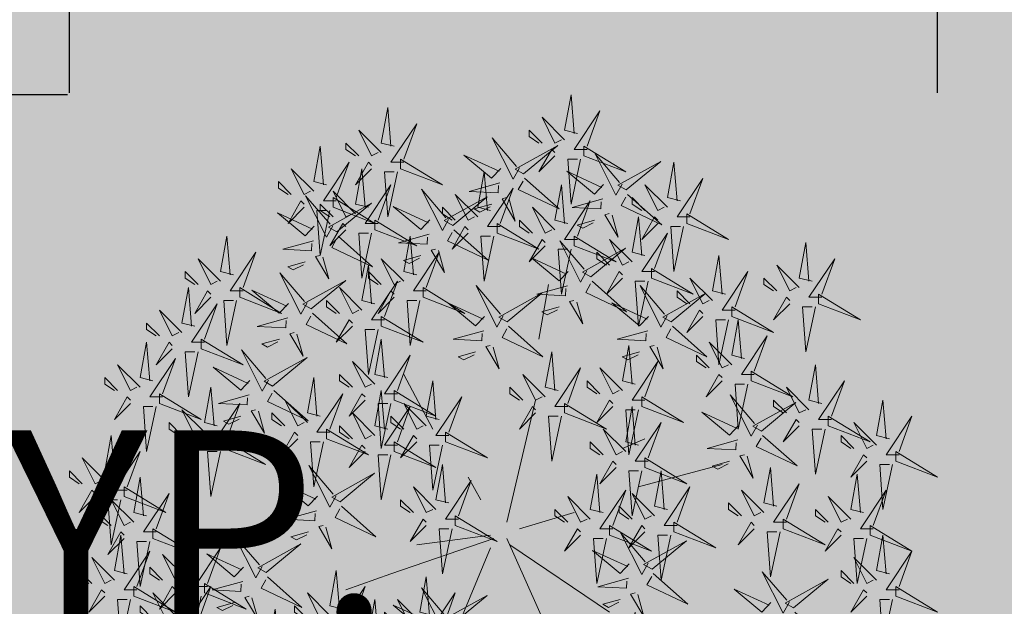
# Model space of a CAD drawing. Units: inches. Extents: x 1704 to 6393, y -157 to 1172.
# Tile 78 of 122: x 2017 to 2048, y 1009 to 1027. Entities that reach past the tile are written whole.
import ezdxf

# ---------------------------------------------------------------- set-up
doc = ezdxf.new("R2010")
doc.units = ezdxf.units.IN
doc.header["$MEASUREMENT"] = 0
doc.layers.add('A-ANNO-DIMS', color=7, linetype='Continuous', lineweight=13)
doc.layers.add('L-shrub', color=74, linetype='Continuous', lineweight=18)
doc.layers.add('L-HRDS-PATT', color=9, linetype='Continuous', lineweight=13, true_color=0xc5c1ba)
doc.styles.get("Standard").update_dxf_attribs({"font": 'arial.ttf'})
doc.dimstyles.get("Standard").update_dxf_attribs({"dimtxt": 6, "dimasz": 2, "dimexe": 0.18, "dimexo": 0.0625, "dimgap": 0.09, "dimtad": 0, "dimtih": 1, "dimtoh": 1, "dimdec": 1, "dimzin": 0, "dimdsep": 46, "dimlunit": 3, "dimtxsty": 'Standard', "dimblk": 'ARCHTICK', "dimcen": 0.09, "dimadec": 0, "dimazin": 0, "dimtfac": 1, "dimtdec": 1, "dimtofl": 0, "dimtmove": 0, "dimatfit": 3, "dimfxl": 1, "dimtolj": 1, "dimtzin": 0, "dimarcsym": 0})

# ---------------------------------------------------------------- blocks, each defined once
blk = doc.blocks.new('autumn shrub')
at = {"layer": 'L-shrub'}
for p, q in [((11.54, 1.92), (51.94, 98)), ((1.92, -3.84), (-38.48, 86.47)), ((-98.12, 69.17), (-107.74, 74.94)), ((0, 0), (-59.64, 40.35)), ((71.18, 17.29), (98.12, 26.9)), ((9.62, -3.84), (71.18, 17.29)), ((11.54, -5.76), (55.79, 0)), ((-5.77, -9.61), (-38.48, -19.21)), ((1.92, -13.45), (-15.39, -86.47)), ((17.31, -26.9), (25.01, -40.35)), ((-76.95, -34.59), (-126.97, -48.04)), ((-67.33, -57.64), (-80.8, -63.41)), ((46.17, -69.17), (63.49, -101.84)), ((-17.31, -122.97), (-23.09, -155.64))]:
    blk.add_line(p, q, dxfattribs=at)
for points in [[(5.77, 222.89), (11.54, 249.79), (13.47, 222.89), (7.7, 222.89)], [(-100.04, 203.68), (-94.27, 230.58), (-92.34, 203.68), (-98.12, 203.68)], [(3.85, 220.97), (-21.16, 230.58), (3.85, 215.21), (3.85, 220.97)], [(21.16, 220.97), (30.78, 230.58), (23.09, 217.13), (21.16, 219.05)], [(98.12, 194.07), (103.89, 220.97), (105.81, 194.07), (100.04, 194.07)], [(1.92, 217.13), (9.62, 217.13), (-5.77, 194.07), (1.92, 215.21)], [(15.39, 211.36), (28.86, 197.91), (21.16, 213.28), (17.31, 211.36)], [(28.86, 213.28), (36.55, 205.6), (36.55, 209.44), (30.78, 213.28)], [(-101.96, 201.75), (-126.97, 211.36), (-101.96, 195.99), (-101.96, 201.75)], [(-84.65, 201.75), (-75.03, 211.36), (-82.73, 197.91), (-84.65, 199.83)], [(-51.51, 194.97), (-55.15, 208.07), (-47.22, 194.76), (-49.84, 194.03)], [(7.7, 207.52), (15.39, 205.6), (11.54, 184.46), (9.62, 207.52)], [(46.17, 180.62), (51.94, 207.52), (53.87, 180.62), (48.1, 180.62)], [(-60.75, 182.51), (-81.34, 200.76), (-56.96, 189.22), (-59.8, 184.19)], [(-41.04, 197.9), (-30.56, 200.83), (-33.91, 202.71), (-40.09, 199.58)], [(96.19, 192.15), (71.18, 201.75), (96.19, 186.38), (96.19, 192.15)], [(113.51, 192.15), (123.13, 201.75), (115.43, 188.3), (113.51, 190.23)], [(-103.89, 197.91), (-96.19, 197.91), (-111.58, 174.85), (-103.89, 195.99)], [(-103.45, 175.76), (-107.1, 188.86), (-99.16, 175.55), (-101.78, 174.81)], [(-90.42, 192.15), (-76.95, 178.7), (-84.65, 194.07), (-88.5, 192.15)], [(-76.95, 194.07), (-69.26, 186.38), (-69.26, 190.23), (-75.03, 194.07)], [(-45.98, 185.23), (-27.65, 190.35), (-44.82, 191.2), (-45.03, 186.9)], [(-98.12, 188.3), (-90.42, 186.38), (-94.27, 165.25), (-96.19, 188.3)], [(-92.98, 178.69), (-82.5, 181.61), (-85.85, 183.5), (-92.03, 180.36)], [(-57.62, 176.33), (-53.83, 183.03), (-41.31, 158.3), (-55.94, 175.38)], [(15.39, 161.4), (21.16, 188.3), (23.09, 161.4), (17.31, 161.4)], [(44.25, 178.7), (19.24, 188.3), (44.25, 172.93), (44.25, 178.7)], [(61.56, 178.7), (71.18, 188.3), (63.49, 174.85), (61.56, 176.78)], [(94.27, 188.3), (101.96, 188.3), (86.57, 165.25), (94.27, 186.38)], [(107.74, 182.54), (121.2, 169.09), (113.51, 184.46), (109.66, 182.54)], [(121.2, 184.46), (128.9, 176.78), (128.9, 180.62), (123.13, 184.46)], [(-112.69, 163.3), (-133.28, 181.54), (-108.91, 170), (-111.74, 164.97)], [(-60.02, 179.89), (-80.67, 162.83), (-55, 177.06), (-60.02, 179.89)], [(-46.41, 176.64), (-40.96, 182.39), (-24.44, 168.66), (-45.47, 178.31)], [(100.04, 178.7), (107.74, 176.78), (103.89, 155.64), (101.96, 178.7)], [(138.52, 155.64), (144.29, 182.54), (146.21, 155.64), (140.44, 155.64)], [(-131.51, 152.18), (-139.33, 153.55), (-136.98, 174.91), (-133.43, 152.04)], [(-97.92, 166.01), (-79.59, 171.13), (-96.76, 171.98), (-96.98, 167.69)], [(42.32, 174.85), (50.02, 174.85), (34.63, 151.8), (42.32, 172.93)], [(55.79, 169.09), (69.26, 155.64), (61.56, 171.01), (57.72, 169.09)], [(69.26, 171.01), (76.95, 163.33), (76.95, 167.17), (71.18, 171.01)], [(-184.69, 138.35), (-178.92, 165.25), (-176.99, 138.35), (-182.77, 138.35)], [(-125.08, 143), (-132.76, 142.46), (-119.03, 166.55), (-125.21, 144.92)], [(-57.28, 154.62), (-60.92, 167.72), (-52.99, 154.41), (-55.61, 153.68)], [(13.47, 159.48), (-11.54, 169.09), (13.47, 153.72), (13.47, 159.48)], [(30.78, 159.48), (40.4, 169.09), (32.71, 155.64), (30.78, 157.56)], [(48.1, 165.25), (55.79, 163.33), (51.94, 142.19), (50.02, 165.25)], [(57.72, 140.27), (63.49, 167.17), (65.41, 140.27), (59.64, 140.27)], [(-138.92, 147.8), (-153.3, 160.27), (-144.54, 145.48), (-140.84, 147.67)], [(-111.96, 160.68), (-132.62, 143.61), (-106.94, 157.85), (-111.96, 160.68)], [(-109.56, 157.11), (-105.78, 163.82), (-93.26, 139.08), (-107.89, 156.17)], [(-98.36, 157.42), (-92.9, 163.18), (-76.38, 149.44), (-97.41, 159.1)], [(-66.52, 142.16), (-87.11, 160.4), (-62.74, 148.86), (-65.57, 143.84)], [(-46.81, 157.55), (-36.33, 160.48), (-39.68, 162.36), (-45.86, 159.22)], [(136.59, 153.72), (111.58, 163.33), (136.59, 147.95), (136.59, 153.72)], [(153.91, 153.72), (163.53, 163.33), (155.83, 149.87), (153.91, 151.8)], [(11.54, 155.64), (19.24, 155.64), (3.85, 132.58), (11.54, 153.72)], [(-152.22, 144.94), (-160.44, 152.06), (-160.16, 148.23), (-154.14, 144.8)], [(-88.06, 135.41), (-91.71, 148.51), (-83.77, 135.2), (-86.39, 134.46)], [(-51.75, 144.88), (-33.42, 150), (-50.59, 150.85), (-50.8, 146.55)], [(25.01, 149.87), (38.48, 136.42), (30.78, 151.8), (26.93, 149.87)], [(55.79, 138.35), (30.78, 147.95), (55.79, 132.58), (55.79, 138.35)], [(38.48, 151.8), (46.17, 144.11), (46.17, 147.95), (40.4, 151.8)], [(73.11, 138.35), (82.73, 147.95), (75.03, 134.5), (73.11, 136.42)], [(134.67, 149.87), (142.36, 149.87), (126.97, 126.82), (134.67, 147.95)], [(150.06, 122.97), (155.83, 149.87), (157.76, 122.97), (151.98, 122.97)], [(-186.61, 136.42), (-211.62, 146.03), (-186.61, 130.66), (-186.61, 136.42)], [(-169.3, 136.42), (-159.68, 146.03), (-167.38, 132.58), (-169.3, 134.5)], [(-144, 137.81), (-152.92, 127.55), (-146.19, 141.51), (-144.13, 139.73)], [(-126.73, 139.03), (-101.1, 131.22), (-127.13, 144.78), (-126.73, 139.03)], [(-77.59, 138.33), (-67.11, 141.26), (-70.46, 143.15), (-76.64, 140.01)], [(-63.39, 135.98), (-59.61, 142.68), (-47.08, 117.95), (-61.71, 135.03)], [(-52.18, 136.28), (-46.73, 142.04), (-30.21, 128.31), (-51.24, 137.96)], [(17.31, 146.03), (25.01, 144.11), (21.16, 122.97), (19.24, 146.03)], [(148.14, 144.11), (161.6, 130.66), (153.91, 146.03), (150.06, 144.11)], [(161.6, 146.03), (169.3, 138.35), (169.3, 142.19), (163.53, 146.03)], [(-128.51, 136.98), (-132.37, 109.74), (-136.19, 136.44), (-130.43, 136.85)], [(-97.3, 122.95), (-117.89, 141.19), (-93.52, 129.65), (-96.35, 124.62)], [(-65.79, 139.54), (-86.44, 122.48), (-60.77, 136.71), (-65.79, 139.54)], [(19.67, 127.72), (16.03, 140.82), (23.96, 127.51), (21.35, 126.78)], [(108.17, 127.72), (104.53, 140.82), (112.46, 127.51), (109.84, 126.78)], [(140.44, 140.27), (148.14, 138.35), (144.29, 117.21), (142.36, 140.27)], [(-188.54, 132.58), (-180.84, 132.58), (-196.23, 109.52), (-188.54, 130.66)], [(-157.32, 118.11), (-160.96, 131.21), (-153.03, 117.9), (-155.65, 117.17)], [(-82.53, 125.66), (-64.2, 130.78), (-81.37, 131.63), (-81.59, 127.34)], [(10.44, 115.26), (-10.16, 133.5), (14.22, 121.96), (11.38, 116.94)], [(30.15, 130.65), (40.62, 133.58), (37.28, 135.46), (31.09, 132.32)], [(53.87, 134.5), (61.56, 134.5), (46.17, 111.45), (53.87, 132.58)], [(67.33, 128.74), (80.8, 115.29), (73.11, 130.66), (69.26, 128.74)], [(98.93, 115.26), (78.34, 133.5), (102.71, 121.96), (99.88, 116.94)], [(78.88, 103.76), (84.65, 130.66), (86.57, 103.76), (80.8, 103.76)], [(80.8, 130.66), (88.5, 122.97), (88.5, 126.82), (82.73, 130.66)], [(118.64, 130.65), (129.12, 133.58), (125.77, 135.46), (119.59, 132.32)], [(148.14, 121.05), (123.13, 130.66), (148.14, 115.29), (148.14, 121.05)], [(165.45, 121.05), (175.07, 130.66), (167.38, 117.21), (165.45, 119.13)], [(-166.56, 105.65), (-187.15, 123.9), (-162.78, 112.36), (-165.61, 107.33)], [(-175.07, 126.82), (-161.6, 113.37), (-169.3, 128.74), (-173.15, 126.82)], [(-161.6, 128.74), (-153.91, 121.05), (-153.91, 124.9), (-159.68, 128.74)], [(-146.85, 121.04), (-136.37, 123.97), (-139.72, 125.86), (-145.9, 122.72)], [(-103.89, 101.84), (-98.12, 128.74), (-96.19, 101.84), (-101.96, 101.84)], [(25.2, 117.98), (43.54, 123.1), (26.37, 123.95), (26.15, 119.65)], [(59.64, 124.9), (67.33, 122.97), (63.49, 101.84), (61.56, 124.9)], [(113.7, 117.98), (132.03, 123.1), (114.86, 123.95), (114.65, 119.65)], [(-182.77, 122.97), (-175.07, 121.05), (-178.92, 99.92), (-180.84, 122.97)], [(-96.57, 120.33), (-117.23, 103.26), (-91.55, 117.49), (-96.57, 120.33)], [(-94.17, 116.76), (-90.39, 123.47), (-77.87, 98.73), (-92.49, 115.82)], [(-82.96, 117.07), (-77.51, 122.83), (-60.99, 109.09), (-82.02, 118.75)], [(-26.93, 94.15), (-21.16, 121.05), (-19.24, 94.15), (-25.01, 94.15)], [(200.08, 94.15), (205.85, 121.05), (207.78, 94.15), (202, 94.15)], [(-151.79, 108.37), (-133.46, 113.49), (-150.63, 114.34), (-150.84, 110.04)], [(11.17, 112.64), (-9.49, 95.58), (16.19, 109.81), (11.17, 112.64)], [(13.57, 109.08), (17.35, 115.78), (29.87, 91.05), (15.24, 108.13)], [(24.77, 109.38), (30.23, 115.14), (46.74, 101.41), (25.72, 111.06)], [(99.66, 112.64), (79.01, 95.58), (104.68, 109.81), (99.66, 112.64)], [(102.06, 109.08), (105.85, 115.78), (118.37, 91.05), (103.74, 108.13)], [(113.27, 109.38), (118.72, 115.14), (135.24, 101.41), (114.21, 111.06)], [(146.21, 117.21), (153.91, 117.21), (138.52, 94.15), (146.21, 115.29)], [(159.68, 111.45), (173.15, 98), (165.45, 113.37), (161.6, 111.45)], [(173.15, 113.37), (180.84, 105.68), (180.84, 109.52), (175.07, 113.37)], [(-184.69, 80.7), (-178.92, 107.6), (-176.99, 80.7), (-182.77, 80.7)], [(-163.43, 99.47), (-159.65, 106.17), (-147.12, 81.44), (-161.75, 98.53)], [(-105.81, 99.92), (-130.82, 109.52), (-105.81, 94.15), (-105.81, 99.92)], [(-88.5, 99.92), (-78.88, 109.52), (-86.57, 96.07), (-88.5, 98)], [(76.95, 101.84), (51.94, 111.45), (76.95, 96.07), (76.95, 101.84)], [(94.27, 101.84), (103.89, 111.45), (96.19, 98), (94.27, 99.92)], [(151.98, 107.6), (159.68, 105.68), (155.83, 84.54), (153.91, 107.6)], [(-165.83, 103.03), (-186.48, 85.97), (-160.81, 100.2), (-165.83, 103.03)], [(-152.22, 99.78), (-146.77, 105.54), (-130.25, 91.8), (-151.28, 101.45)], [(-134.24, 89.29), (-137.88, 102.39), (-129.94, 89.08), (-132.56, 88.35)], [(-80.8, 78.78), (-75.03, 105.68), (-73.11, 78.78), (-78.88, 78.78)], [(-28.86, 92.23), (-53.87, 101.84), (-28.86, 86.47), (-28.86, 92.23)], [(-11.54, 92.23), (-1.92, 101.84), (-9.62, 88.39), (-11.54, 90.31)], [(134.67, 76.86), (140.44, 103.76), (142.36, 76.86), (136.59, 76.86)], [(198.16, 92.23), (173.15, 101.84), (198.16, 86.47), (198.16, 92.23)], [(215.47, 92.23), (225.09, 101.84), (217.4, 88.39), (215.47, 90.31)], [(-143.47, 76.83), (-164.07, 95.07), (-139.69, 83.53), (-142.53, 78.51)], [(-123.76, 92.22), (-113.29, 95.15), (-116.63, 97.03), (-122.82, 93.89)], [(-107.74, 96.07), (-100.04, 96.07), (-115.43, 73.02), (-107.74, 94.15)], [(75.03, 98), (82.73, 98), (67.33, 74.94), (75.03, 96.07)], [(75.03, 71.09), (80.8, 98), (82.73, 71.09), (76.95, 71.09)], [(-186.61, 78.78), (-211.62, 88.39), (-186.61, 73.02), (-186.61, 78.78)], [(-169.3, 78.78), (-159.68, 88.39), (-167.38, 74.94), (-169.3, 76.86)], [(-94.27, 90.31), (-80.8, 76.86), (-88.5, 92.23), (-92.34, 90.31)], [(-80.8, 92.23), (-73.11, 84.54), (-73.11, 88.39), (-78.88, 92.23)], [(-30.78, 88.39), (-23.09, 88.39), (-38.48, 65.33), (-30.78, 86.47)], [(80.8, 88.39), (88.5, 86.47), (84.65, 65.33), (82.73, 88.39)], [(88.5, 92.23), (101.96, 78.78), (94.27, 94.15), (90.42, 92.23)], [(101.96, 94.15), (109.66, 86.47), (109.66, 90.31), (103.89, 94.15)], [(196.23, 88.39), (203.93, 88.39), (188.54, 65.33), (196.23, 86.47)], [(-128.7, 79.55), (-110.37, 84.67), (-127.54, 85.52), (-127.76, 81.22)], [(-82.73, 76.86), (-107.74, 86.47), (-82.73, 71.09), (-82.73, 76.86)], [(-101.96, 86.47), (-94.27, 84.54), (-98.12, 63.41), (-100.04, 86.47)], [(-65.41, 76.86), (-55.79, 86.47), (-63.49, 73.02), (-65.41, 74.94)], [(-17.31, 82.62), (-3.85, 69.17), (-11.54, 84.54), (-15.39, 82.62)], [(-3.85, 84.54), (3.85, 76.86), (3.85, 80.7), (-1.92, 84.54)], [(44.25, 57.64), (50.02, 84.54), (51.94, 57.64), (46.17, 57.64)], [(132.75, 74.94), (107.74, 84.54), (132.75, 69.17), (132.75, 74.94)], [(150.06, 74.94), (159.68, 84.54), (151.98, 71.09), (150.06, 73.02)], [(209.7, 82.62), (223.17, 69.17), (215.47, 84.54), (211.62, 82.62)], [(223.17, 84.54), (230.86, 76.86), (230.86, 80.7), (225.09, 84.54)], [(-140.34, 70.65), (-136.56, 77.35), (-124.04, 52.62), (-138.67, 69.7)], [(-129.14, 70.95), (-123.68, 76.71), (-107.16, 62.98), (-128.19, 72.63)], [(-25.01, 78.78), (-17.31, 76.86), (-21.16, 55.72), (-23.09, 78.78)], [(73.11, 69.17), (48.1, 78.78), (73.11, 63.41), (73.11, 69.17)], [(90.42, 69.17), (100.04, 78.78), (92.34, 65.33), (90.42, 67.25)], [(98.12, 53.8), (103.89, 80.7), (105.81, 53.8), (100.04, 53.8)], [(190.46, 53.8), (196.23, 80.7), (198.16, 53.8), (192.39, 53.8)], [(202, 78.78), (209.7, 76.86), (205.85, 55.72), (203.93, 78.78)], [(-188.54, 74.94), (-180.84, 74.94), (-196.23, 51.88), (-188.54, 73.02)], [(-175.07, 69.17), (-161.6, 55.72), (-169.3, 71.09), (-173.15, 69.17)], [(-142.74, 74.21), (-163.4, 57.15), (-137.72, 71.38), (-142.74, 74.21)], [(-161.6, 71.09), (-153.91, 63.41), (-153.91, 67.25), (-159.68, 71.09)], [(-84.65, 73.02), (-76.95, 73.02), (-92.34, 49.96), (-84.65, 71.09)], [(42.76, 62.39), (39.12, 75.49), (47.05, 62.18), (44.43, 61.45)], [(130.82, 71.09), (138.52, 71.09), (123.13, 48.04), (130.82, 69.17)], [(-182.77, 65.33), (-175.07, 63.41), (-178.92, 42.27), (-180.84, 65.33)], [(-161.17, 52.78), (-164.81, 65.88), (-156.88, 52.57), (-159.5, 51.84)], [(-71.18, 67.25), (-57.72, 53.8), (-65.41, 69.17), (-69.26, 67.25)], [(-57.72, 69.17), (-50.02, 61.49), (-50.02, 65.33), (-55.79, 69.17)], [(33.52, 49.93), (12.93, 68.17), (37.3, 56.63), (34.47, 51.61)], [(42.32, 55.72), (17.31, 65.33), (42.32, 49.96), (42.32, 55.72)], [(53.23, 65.32), (63.71, 68.25), (60.36, 70.13), (54.18, 66.99)], [(59.64, 55.72), (69.26, 65.33), (61.56, 51.88), (59.64, 53.8)], [(71.18, 65.33), (78.88, 65.33), (63.49, 42.27), (71.18, 63.41)], [(144.29, 65.33), (157.76, 51.88), (150.06, 67.25), (146.21, 65.33)], [(157.76, 67.25), (165.45, 59.57), (165.45, 63.41), (159.68, 67.25)], [(-228.94, 32.67), (-223.17, 59.57), (-221.24, 32.67), (-227.01, 32.67)], [(-150.69, 55.71), (-140.22, 58.64), (-143.57, 60.53), (-149.75, 57.39)], [(-78.88, 63.41), (-71.18, 61.49), (-75.03, 40.35), (-76.95, 63.41)], [(96.19, 51.88), (71.18, 61.49), (96.19, 46.12), (96.19, 51.88)], [(84.65, 59.57), (98.12, 46.12), (90.42, 61.49), (86.57, 59.57)], [(98.12, 61.49), (105.81, 53.8), (105.81, 57.64), (100.04, 61.49)], [(113.51, 51.88), (123.13, 61.49), (115.43, 48.04), (113.51, 49.96)], [(136.59, 61.49), (144.29, 59.57), (140.44, 38.43), (138.52, 61.49)], [(188.54, 51.88), (163.53, 61.49), (188.54, 46.12), (188.54, 51.88)], [(205.85, 51.88), (215.47, 61.49), (207.78, 48.04), (205.85, 49.96)], [(227.01, 32.67), (232.79, 59.57), (234.71, 32.67), (228.94, 32.67)], [(-170.4, 40.32), (-191, 58.57), (-166.62, 47.03), (-169.46, 42)], [(48.29, 52.64), (66.62, 57.77), (49.45, 58.62), (49.24, 54.32)], [(76.95, 55.72), (84.65, 53.8), (80.8, 32.67), (78.88, 55.72)], [(184.69, 30.74), (190.46, 57.64), (192.39, 30.74), (186.61, 30.74)], [(-155.64, 43.04), (-137.31, 48.16), (-154.48, 49.01), (-154.69, 44.71)], [(34.25, 47.31), (13.6, 30.25), (39.27, 44.48), (34.25, 47.31)], [(40.4, 51.88), (48.1, 51.88), (32.71, 28.82), (40.4, 49.96)], [(36.65, 43.75), (40.43, 50.45), (52.96, 25.72), (38.33, 42.8)], [(47.86, 44.05), (53.31, 49.81), (69.83, 36.08), (48.8, 45.73)], [(53.87, 46.12), (67.33, 32.67), (59.64, 48.04), (55.79, 46.12)], [(67.33, 48.04), (75.03, 40.35), (75.03, 44.19), (69.26, 48.04)], [(94.27, 48.04), (101.96, 48.04), (86.57, 24.98), (94.27, 46.12)], [(186.61, 48.04), (194.31, 48.04), (178.92, 24.98), (186.61, 46.12)], [(-76.52, 29.73), (-80.16, 42.83), (-72.23, 29.51), (-74.85, 28.78)], [(46.17, 42.27), (53.87, 40.35), (50.02, 19.21), (48.1, 42.27)], [(107.74, 42.27), (121.2, 28.82), (113.51, 44.19), (109.66, 42.27)], [(121.2, 44.19), (128.9, 36.51), (128.9, 40.35), (123.13, 44.19)], [(154.34, 31.65), (150.7, 44.75), (158.63, 31.44), (156.02, 30.7)], [(200.08, 42.27), (213.55, 28.82), (205.85, 44.19), (202, 42.27)], [(213.55, 44.19), (221.24, 36.51), (221.24, 40.35), (215.47, 44.19)], [(-230.86, 30.74), (-255.87, 40.35), (-230.86, 24.98), (-230.86, 30.74)], [(-213.55, 30.74), (-203.93, 40.35), (-211.62, 26.9), (-213.55, 28.82)], [(-169.68, 37.7), (-190.33, 20.64), (-164.66, 34.87), (-169.68, 37.7)], [(-167.27, 34.14), (-163.49, 40.84), (-150.97, 16.11), (-165.6, 33.2)], [(-156.07, 34.45), (-150.62, 40.21), (-134.1, 26.47), (-155.13, 36.12)], [(-85.76, 17.27), (-106.35, 35.51), (-81.97, 23.97), (-84.81, 18.94)], [(-66.05, 32.65), (-55.57, 35.58), (-58.92, 37.47), (-65.1, 34.33)], [(100.04, 38.43), (107.74, 36.51), (103.89, 15.37), (101.96, 38.43)], [(145.11, 19.19), (124.51, 37.43), (148.89, 25.89), (146.05, 20.86)], [(182.77, 28.82), (157.76, 38.43), (182.77, 23.06), (182.77, 28.82)], [(164.82, 34.57), (175.29, 37.5), (171.94, 39.39), (165.76, 36.25)], [(192.39, 38.43), (200.08, 36.51), (196.23, 15.37), (194.31, 38.43)], [(225.09, 30.74), (200.08, 40.35), (225.09, 24.98), (225.09, 30.74)], [(200.08, 28.82), (209.7, 38.43), (202, 24.98), (200.08, 26.9)], [(242.41, 30.74), (252.02, 40.35), (244.33, 26.9), (242.41, 28.82)], [(-232.79, 26.9), (-225.09, 26.9), (-240.48, 3.84), (-232.79, 24.98)], [(-70.99, 19.98), (-52.66, 25.1), (-69.83, 25.95), (-70.04, 21.66)], [(159.87, 21.9), (178.21, 27.02), (161.04, 27.87), (160.82, 23.58)], [(180.84, 24.98), (188.54, 24.98), (173.15, 1.92), (180.84, 23.06)], [(223.17, 26.9), (230.86, 26.9), (215.47, 3.84), (223.17, 24.98)], [(215.47, -1.92), (221.24, 24.98), (223.17, -1.92), (217.4, -1.92)], [(-219.32, 21.14), (-205.85, 7.69), (-213.55, 23.06), (-217.4, 21.14)], [(-213.55, -3.84), (-207.78, 23.06), (-205.85, -3.84), (-211.62, -3.84)], [(-205.85, 23.06), (-198.16, 15.37), (-198.16, 19.21), (-203.93, 23.06)], [(-161.6, -7.69), (-155.83, 19.21), (-153.91, -7.69), (-159.68, -7.69)], [(-96.19, -5.76), (-90.42, 21.14), (-88.5, -5.76), (-94.27, -5.76)], [(-82.63, 11.08), (-78.84, 17.78), (-66.32, -6.95), (-80.95, 10.14)], [(-57.72, -3.84), (-51.94, 23.06), (-50.02, -3.84), (-55.79, -3.84)], [(148.24, 13), (152.02, 19.71), (164.54, -5.03), (149.91, 12.06)], [(159.44, 13.31), (164.89, 19.07), (181.41, 5.33), (160.39, 14.99)], [(194.31, 19.21), (207.78, 5.76), (200.08, 21.14), (196.23, 19.21)], [(207.78, 21.14), (215.47, 13.45), (215.47, 17.29), (209.7, 21.14)], [(236.63, 21.14), (250.1, 7.69), (242.41, 23.06), (238.56, 21.14)], [(250.1, 23.06), (257.8, 15.37), (257.8, 19.21), (252.02, 23.06)], [(-227.01, 17.29), (-219.32, 15.37), (-223.17, -5.76), (-225.09, 17.29)], [(-85.03, 14.65), (-105.68, -2.42), (-80.01, 11.81), (-85.03, 14.65)], [(-71.42, 11.39), (-65.97, 17.15), (-49.45, 3.41), (-70.48, 13.06)], [(34.63, -9.61), (40.4, 17.29), (42.32, -9.61), (36.55, -9.61)], [(145.83, 16.57), (125.18, -0.5), (150.86, 13.74), (145.83, 16.57)], [(186.61, 15.37), (194.31, 13.45), (190.46, -7.69), (188.54, 15.37)], [(228.94, 17.29), (236.63, 15.37), (232.79, -5.76), (230.86, 17.29)], [(-215.47, -5.76), (-240.48, 3.84), (-215.47, -11.53), (-215.47, -5.76)], [(-198.16, -5.76), (-188.54, 3.84), (-196.23, -9.61), (-198.16, -7.69)], [(-163.53, -9.61), (-188.54, 0), (-163.53, -15.37), (-163.53, -9.61)], [(-146.21, -9.61), (-136.59, 0), (-144.29, -13.45), (-146.21, -11.53)], [(-98.12, -7.69), (-123.13, 1.92), (-98.12, -13.45), (-98.12, -7.69)], [(-59.64, -5.76), (-84.65, 3.84), (-59.64, -11.53), (-59.64, -5.76)], [(-80.8, -7.69), (-71.18, 1.92), (-78.88, -11.53), (-80.8, -9.61)], [(-42.32, -5.76), (-32.71, 3.84), (-40.4, -9.61), (-42.32, -7.69)], [(110.09, -10.62), (106.45, 2.47), (114.39, -10.84), (111.77, -11.57)], [(213.55, -3.84), (188.54, 5.76), (213.55, -9.61), (213.55, -3.84)], [(230.86, -3.84), (240.48, 5.76), (232.79, -7.69), (230.86, -5.76)], [(232.79, -26.9), (238.56, 0), (240.48, -26.9), (234.71, -26.9)], [(32.71, -11.53), (7.7, -1.92), (32.71, -17.29), (32.71, -11.53)], [(50.02, -11.53), (59.64, -1.92), (51.94, -15.37), (50.02, -13.45)], [(100.86, -23.09), (80.26, -4.84), (104.64, -16.38), (101.8, -21.41)], [(120.57, -7.7), (131.04, -4.77), (127.7, -2.88), (121.51, -6.02)], [(-217.4, -9.61), (-209.7, -9.61), (-225.09, -32.67), (-217.4, -11.53)], [(-100.04, -11.53), (-92.34, -11.53), (-107.74, -34.59), (-100.04, -13.45)], [(-61.56, -9.61), (-53.87, -9.61), (-69.26, -32.67), (-61.56, -11.53)], [(211.62, -7.69), (219.32, -7.69), (203.93, -30.74), (211.62, -9.61)], [(225.09, -13.45), (238.56, -26.9), (230.86, -11.53), (227.01, -13.45)], [(238.56, -11.53), (246.25, -19.21), (246.25, -15.37), (240.48, -11.53)], [(-203.93, -15.37), (-190.46, -28.82), (-198.16, -13.45), (-202, -15.37)], [(-190.46, -13.45), (-182.77, -21.14), (-182.77, -17.29), (-188.54, -13.45)], [(-165.45, -13.45), (-157.76, -13.45), (-173.15, -36.51), (-165.45, -15.37)], [(-151.98, -19.21), (-138.52, -32.67), (-146.21, -17.29), (-150.06, -19.21)], [(-138.52, -17.29), (-130.82, -24.98), (-130.82, -21.14), (-136.59, -17.29)], [(-86.57, -17.29), (-73.11, -30.74), (-80.8, -15.37), (-84.65, -17.29)], [(-78.88, -44.19), (-73.11, -17.29), (-71.18, -44.19), (-76.95, -44.19)], [(-73.11, -15.37), (-65.41, -23.06), (-65.41, -19.21), (-71.18, -15.37)], [(-48.1, -15.37), (-34.63, -28.82), (-42.32, -13.45), (-46.17, -15.37)], [(-34.63, -13.45), (-26.93, -21.14), (-26.93, -17.29), (-32.71, -13.45)], [(30.78, -15.37), (38.48, -15.37), (23.09, -38.43), (30.78, -17.29)], [(115.63, -20.37), (133.96, -15.25), (116.79, -14.4), (116.57, -18.7)], [(217.4, -17.29), (225.09, -19.21), (221.24, -40.35), (219.32, -17.29)], [(-228.94, -48.04), (-223.17, -21.14), (-221.24, -48.04), (-227.01, -48.04)], [(-211.62, -19.21), (-203.93, -21.14), (-207.78, -42.27), (-209.7, -19.21)], [(-159.68, -23.06), (-151.98, -24.98), (-155.83, -46.12), (-157.76, -23.06)], [(-94.27, -21.14), (-86.57, -23.06), (-90.42, -44.19), (-92.34, -21.14)], [(-55.79, -19.21), (-48.1, -21.14), (-51.94, -42.27), (-53.87, -19.21)], [(44.25, -21.14), (57.72, -34.59), (50.02, -19.21), (46.17, -21.14)], [(57.72, -19.21), (65.41, -26.9), (65.41, -23.06), (59.64, -19.21)], [(103.99, -29.27), (107.77, -22.57), (120.29, -47.3), (105.66, -30.21)], [(115.19, -28.96), (120.65, -23.2), (137.17, -36.94), (116.14, -27.29)], [(230.86, -28.82), (205.85, -19.21), (230.86, -34.59), (230.86, -28.82)], [(248.18, -28.82), (257.8, -19.21), (250.1, -32.67), (248.18, -30.74)], [(36.55, -24.98), (44.25, -26.9), (40.4, -48.04), (38.48, -24.98)], [(71.18, -53.8), (76.95, -26.9), (78.88, -53.8), (73.11, -53.8)], [(101.59, -25.71), (80.93, -42.77), (106.61, -28.54), (101.59, -25.71)], [(173.15, -55.72), (178.92, -28.82), (180.84, -55.72), (175.07, -55.72)], [(40.4, -59.57), (46.17, -32.67), (48.1, -59.57), (42.32, -59.57)], [(111.58, -61.49), (117.35, -34.59), (119.28, -61.49), (113.51, -61.49)], [(228.94, -32.67), (236.63, -32.67), (221.24, -55.72), (228.94, -34.59)], [(-230.86, -49.96), (-255.87, -40.35), (-230.86, -55.72), (-230.86, -49.96)], [(-213.55, -49.96), (-203.93, -40.35), (-211.62, -53.8), (-213.55, -51.88)], [(-141.93, -52.9), (-145.57, -39.8), (-137.64, -53.11), (-140.26, -53.84)], [(-80.8, -46.12), (-105.81, -36.51), (-80.8, -51.88), (-80.8, -46.12)], [(-63.49, -46.12), (-53.87, -36.51), (-61.56, -49.96), (-63.49, -48.04)], [(242.41, -38.43), (255.87, -51.88), (248.18, -36.51), (244.33, -38.43)], [(255.87, -36.51), (263.57, -44.19), (263.57, -40.35), (257.8, -36.51)], [(-188.54, -69.17), (-182.77, -42.27), (-180.84, -69.17), (-186.61, -69.17)], [(-151.17, -65.36), (-171.76, -47.11), (-147.39, -58.66), (-150.22, -63.68)], [(-131.46, -49.97), (-120.98, -47.04), (-124.33, -45.16), (-130.51, -48.29)], [(69.26, -55.72), (44.25, -46.12), (69.26, -61.49), (69.26, -55.72)], [(86.57, -55.72), (96.19, -46.12), (88.5, -59.57), (86.57, -57.64)], [(234.71, -42.27), (242.41, -44.19), (238.56, -65.33), (236.63, -42.27)], [(-82.73, -49.96), (-75.03, -49.96), (-90.42, -73.02), (-82.73, -51.88)], [(-30.78, -76.86), (-25.01, -49.96), (-23.09, -76.86), (-28.86, -76.86)], [(38.48, -61.49), (13.47, -51.88), (38.48, -67.25), (38.48, -61.49)], [(55.79, -61.49), (65.41, -51.88), (57.72, -65.33), (55.79, -63.41)], [(171.22, -57.64), (146.21, -48.04), (171.22, -63.41), (171.22, -57.64)], [(188.54, -57.64), (198.16, -48.04), (190.46, -61.49), (188.54, -59.57)], [(-232.79, -53.8), (-225.09, -53.8), (-240.48, -76.86), (-232.79, -55.72)], [(-219.32, -59.57), (-205.85, -73.02), (-213.55, -57.64), (-217.4, -59.57)], [(-205.85, -57.64), (-198.16, -65.33), (-198.16, -61.49), (-203.93, -57.64)], [(-136.4, -62.64), (-118.07, -57.52), (-135.24, -56.67), (-135.45, -60.97)], [(-76.95, -80.7), (-71.18, -53.8), (-69.26, -80.7), (-75.03, -80.7)], [(-69.26, -55.72), (-55.79, -69.17), (-63.49, -53.8), (-67.33, -55.72)], [(-55.79, -53.8), (-48.1, -61.49), (-48.1, -57.64), (-53.87, -53.8)], [(71.18, -84.54), (76.95, -57.64), (78.88, -84.54), (73.11, -84.54)], [(109.66, -63.41), (84.65, -53.8), (109.66, -69.17), (109.66, -63.41)], [(126.97, -63.41), (136.59, -53.8), (128.9, -67.25), (126.97, -65.33)], [(211.62, -82.62), (217.4, -55.72), (219.32, -82.62), (213.55, -82.62)], [(-227.01, -63.41), (-219.32, -65.33), (-223.17, -86.47), (-225.09, -63.41)], [(-190.46, -71.09), (-215.47, -61.49), (-190.46, -76.86), (-190.46, -71.09)], [(-173.15, -71.09), (-163.53, -61.49), (-171.22, -74.94), (-173.15, -73.02)], [(-76.95, -59.57), (-69.26, -61.49), (-73.11, -82.62), (-75.03, -59.57)], [(67.33, -59.57), (75.03, -59.57), (59.64, -82.62), (67.33, -61.49)], [(80.8, -65.33), (94.27, -78.78), (86.57, -63.41), (82.73, -65.33)], [(94.27, -63.41), (101.96, -71.09), (101.96, -67.25), (96.19, -63.41)], [(169.3, -61.49), (176.99, -61.49), (161.6, -84.54), (169.3, -63.41)], [(-150.44, -67.98), (-171.09, -85.04), (-145.42, -70.81), (-150.44, -67.98)], [(-148.04, -71.54), (-144.26, -64.84), (-131.73, -89.57), (-146.36, -72.49)], [(-142.36, -96.07), (-136.59, -69.17), (-134.67, -96.07), (-140.44, -96.07)], [(-136.83, -71.23), (-131.38, -65.48), (-114.86, -79.21), (-135.89, -69.56)], [(-32.71, -78.78), (-57.72, -69.17), (-32.71, -84.54), (-32.71, -78.78)], [(-15.39, -78.78), (-5.77, -69.17), (-13.47, -82.62), (-15.39, -80.7)], [(36.55, -65.33), (44.25, -65.33), (28.86, -88.39), (36.55, -67.25)], [(50.02, -71.09), (63.49, -84.54), (55.79, -69.17), (51.94, -71.09)], [(63.49, -69.17), (71.18, -76.86), (71.18, -73.02), (65.41, -69.17)], [(73.11, -69.17), (80.8, -71.09), (76.95, -92.23), (75.03, -69.17)], [(107.74, -67.25), (115.43, -67.25), (100.04, -90.31), (107.74, -69.17)], [(150.49, -79.8), (146.85, -66.7), (154.79, -80.01), (152.17, -80.74)], [(182.77, -67.25), (196.23, -80.7), (188.54, -65.33), (184.69, -67.25)], [(196.23, -65.33), (203.93, -73.02), (203.93, -69.17), (198.16, -65.33)], [(-192.39, -74.94), (-184.69, -74.94), (-200.08, -98), (-192.39, -76.86)], [(-78.88, -82.62), (-103.89, -73.02), (-78.88, -88.39), (-78.88, -82.62)], [(-61.56, -82.62), (-51.94, -73.02), (-59.64, -86.47), (-61.56, -84.54)], [(42.32, -74.94), (50.02, -76.86), (46.17, -98), (44.25, -74.94)], [(141.26, -92.26), (120.66, -74.02), (145.04, -85.56), (142.2, -90.58)], [(121.2, -73.02), (134.67, -86.47), (126.97, -71.09), (123.13, -73.02)], [(134.67, -71.09), (142.36, -78.78), (142.36, -74.94), (136.59, -71.09)], [(160.97, -76.87), (171.44, -73.94), (168.1, -72.06), (161.91, -75.19)], [(175.07, -71.09), (182.77, -73.02), (178.92, -94.15), (176.99, -71.09)], [(209.7, -84.54), (184.69, -74.94), (209.7, -90.31), (209.7, -84.54)], [(227.01, -84.54), (236.63, -74.94), (228.94, -88.39), (227.01, -86.47)], [(-178.92, -80.7), (-165.45, -94.15), (-173.15, -78.78), (-176.99, -80.7)], [(-165.45, -78.78), (-157.76, -86.47), (-157.76, -82.62), (-163.53, -78.78)], [(69.26, -86.47), (44.25, -76.86), (69.26, -92.23), (69.26, -86.47)], [(86.57, -86.47), (96.19, -76.86), (88.5, -90.31), (86.57, -88.39)], [(113.51, -76.86), (121.2, -78.78), (117.35, -99.92), (115.43, -76.86)], [(-186.61, -84.54), (-178.92, -86.47), (-182.77, -107.6), (-184.69, -84.54)], [(-80.8, -86.47), (-73.11, -86.47), (-88.5, -109.52), (-80.8, -88.39)], [(-34.63, -82.62), (-26.93, -82.62), (-42.32, -105.68), (-34.63, -84.54)], [(-21.16, -88.39), (-7.7, -101.84), (-15.39, -86.47), (-19.24, -88.39)], [(-7.7, -86.47), (0, -94.15), (0, -90.31), (-5.77, -86.47)], [(156.03, -89.54), (174.36, -84.42), (157.19, -83.57), (156.97, -87.87)], [(-144.29, -98), (-169.3, -88.39), (-144.29, -103.76), (-144.29, -98)], [(-126.97, -98), (-117.35, -88.39), (-125.05, -101.84), (-126.97, -99.92)], [(-67.33, -92.23), (-53.87, -105.68), (-61.56, -90.31), (-65.41, -92.23)], [(-53.87, -90.31), (-46.17, -98), (-46.17, -94.15), (-51.94, -90.31)], [(-28.86, -92.23), (-21.16, -94.15), (-25.01, -115.29), (-26.93, -92.23)], [(67.33, -90.31), (75.03, -90.31), (59.64, -113.37), (67.33, -92.23)], [(80.8, -96.07), (94.27, -109.52), (86.57, -94.15), (82.73, -96.07)], [(94.27, -94.15), (101.96, -101.84), (101.96, -98), (96.19, -94.15)], [(144.39, -98.44), (148.17, -91.74), (160.69, -116.47), (146.06, -99.39)], [(155.59, -98.13), (161.05, -92.38), (177.57, -106.11), (156.54, -96.46)], [(186.61, -115.29), (192.39, -88.39), (194.31, -115.29), (188.54, -115.29)], [(207.78, -88.39), (215.47, -88.39), (200.08, -111.45), (207.78, -90.31)], [(221.24, -94.15), (234.71, -107.6), (227.01, -92.23), (223.17, -94.15)], [(234.71, -92.23), (242.41, -99.92), (242.41, -96.07), (236.63, -92.23)], [(-75.03, -96.07), (-67.33, -98), (-71.18, -119.13), (-73.11, -96.07)], [(73.11, -99.92), (80.8, -101.84), (76.95, -122.97), (75.03, -99.92)], [(141.99, -94.88), (121.33, -111.94), (147.01, -97.71), (141.99, -94.88)], [(213.55, -98), (221.24, -99.92), (217.4, -121.05), (215.47, -98)], [(-146.21, -101.84), (-138.52, -101.84), (-153.91, -124.9), (-146.21, -103.76)], [(-132.75, -107.6), (-119.28, -121.05), (-126.97, -105.68), (-130.82, -107.6)], [(-119.28, -105.68), (-111.58, -113.37), (-111.58, -109.52), (-117.35, -105.68)], [(-88.06, -118.23), (-91.71, -105.13), (-83.77, -118.44), (-86.39, -119.17)], [(10.05, -118.23), (6.41, -105.13), (14.35, -118.44), (11.73, -119.17)], [(78.88, -128.74), (84.65, -101.84), (86.57, -128.74), (80.8, -128.74)], [(-140.44, -111.45), (-132.75, -113.37), (-136.59, -134.5), (-138.52, -111.45)], [(-130.82, -134.5), (-125.05, -107.6), (-123.13, -134.5), (-128.9, -134.5)], [(-77.59, -115.3), (-67.11, -112.37), (-70.46, -110.49), (-76.64, -113.62)], [(20.53, -115.3), (31, -112.37), (27.66, -110.49), (21.47, -113.62)], [(184.69, -117.21), (159.68, -107.6), (184.69, -122.97), (184.69, -117.21)], [(202, -117.21), (211.62, -107.6), (203.93, -121.05), (202, -119.13)], [(-182.77, -142.19), (-176.99, -115.29), (-175.07, -142.19), (-180.84, -142.19)], [(-97.3, -130.69), (-117.89, -112.44), (-93.52, -123.99), (-96.35, -129.01)], [(0.82, -130.69), (-19.78, -112.44), (4.6, -123.99), (1.76, -129.01)], [(127.41, -125.91), (123.77, -112.81), (131.7, -126.12), (129.08, -126.86)], [(-82.53, -127.97), (-64.2, -122.85), (-81.37, -122), (-81.59, -126.3)], [(15.59, -127.97), (33.92, -122.85), (16.75, -122), (16.53, -126.3)], [(76.95, -130.66), (51.94, -121.05), (76.95, -136.42), (76.95, -130.66)], [(53.87, -146.03), (59.64, -119.13), (61.56, -146.03), (55.79, -146.03)], [(94.27, -130.66), (103.89, -121.05), (96.19, -134.5), (94.27, -132.58)], [(118.17, -138.37), (97.58, -120.13), (121.95, -131.67), (119.12, -136.7)], [(137.88, -122.99), (148.36, -120.06), (145.01, -118.17), (138.83, -121.31)], [(163.53, -146.03), (169.3, -119.13), (171.22, -146.03), (165.45, -146.03)], [(182.77, -121.05), (190.46, -121.05), (175.07, -144.11), (182.77, -122.97)], [(-132.75, -136.42), (-157.76, -126.82), (-132.75, -142.19), (-132.75, -136.42)], [(-115.43, -136.42), (-105.81, -126.82), (-113.51, -140.27), (-115.43, -138.35)], [(196.23, -126.82), (209.7, -140.27), (202, -124.9), (198.16, -126.82)], [(209.7, -124.9), (217.4, -132.58), (217.4, -128.74), (211.62, -124.9)], [(-184.69, -144.11), (-209.7, -134.5), (-184.69, -149.87), (-184.69, -144.11)], [(-167.38, -144.11), (-157.76, -134.5), (-165.45, -147.95), (-167.38, -146.03)], [(-96.57, -133.31), (-117.23, -150.37), (-91.55, -136.14), (-96.57, -133.31)], [(-94.17, -136.87), (-90.39, -130.17), (-77.87, -154.9), (-92.49, -137.82)], [(-82.96, -136.56), (-77.51, -130.81), (-60.99, -144.54), (-82.02, -134.89)], [(-82.73, -157.56), (-76.95, -130.66), (-75.03, -157.56), (-80.8, -157.56)], [(-39.97, -145.13), (-43.61, -132.03), (-35.67, -145.34), (-38.29, -146.07)], [(1.55, -133.31), (-19.11, -150.37), (6.57, -136.14), (1.55, -133.31)], [(3.95, -136.87), (7.73, -130.17), (20.25, -154.9), (5.62, -137.82)], [(15.15, -136.56), (20.61, -130.81), (37.13, -144.54), (16.1, -134.89)], [(75.03, -134.5), (82.73, -134.5), (67.33, -157.56), (75.03, -136.42)], [(132.94, -135.66), (151.27, -130.54), (134.1, -129.69), (133.89, -133.98)], [(188.54, -130.66), (196.23, -132.58), (192.39, -153.72), (190.46, -130.66)], [(-134.67, -140.27), (-126.97, -140.27), (-142.36, -163.33), (-134.67, -142.19)], [(-49.2, -157.59), (-69.8, -139.35), (-45.42, -150.89), (-48.26, -155.91)], [(-29.49, -142.2), (-19.02, -139.27), (-22.36, -137.39), (-28.55, -140.52)], [(51.94, -147.95), (26.93, -138.35), (51.94, -153.72), (51.94, -147.95)], [(69.26, -147.95), (78.88, -138.35), (71.18, -151.8), (69.26, -149.87)], [(88.5, -140.27), (101.96, -153.72), (94.27, -138.35), (90.42, -140.27)], [(118.9, -140.99), (98.25, -158.06), (123.92, -143.83), (118.9, -140.99)], [(101.96, -138.35), (109.66, -146.03), (109.66, -142.19), (103.89, -138.35)], [(121.3, -144.56), (125.08, -137.85), (137.61, -162.59), (122.98, -145.5)], [(132.51, -144.25), (137.96, -138.49), (154.48, -152.23), (133.45, -142.57)], [(161.6, -147.95), (136.59, -138.35), (161.6, -153.72), (161.6, -147.95)], [(178.92, -147.95), (188.54, -138.35), (180.84, -151.8), (178.92, -149.87)], [(-121.2, -146.03), (-107.74, -159.48), (-115.43, -144.11), (-119.28, -146.03)], [(-107.74, -144.11), (-100.04, -151.8), (-100.04, -147.95), (-105.81, -144.11)], [(80.8, -144.11), (88.5, -146.03), (84.65, -167.17), (82.73, -144.11)], [(-186.61, -147.95), (-178.92, -147.95), (-194.31, -171.01), (-186.61, -149.87)], [(-173.15, -153.72), (-159.68, -167.17), (-167.38, -151.8), (-171.22, -153.72)], [(-159.68, -151.8), (-151.98, -159.48), (-151.98, -155.64), (-157.76, -151.8)], [(-128.9, -149.87), (-121.2, -151.8), (-125.05, -172.93), (-126.97, -149.87)], [(-84.65, -159.48), (-109.66, -149.87), (-84.65, -165.25), (-84.65, -159.48)], [(-67.33, -159.48), (-57.72, -149.87), (-65.41, -163.33), (-67.33, -161.4)], [(-36.55, -176.78), (-30.78, -149.87), (-28.86, -176.78), (-34.63, -176.78)], [(-34.43, -154.87), (-16.1, -149.75), (-33.27, -148.9), (-33.49, -153.2)], [(50.02, -151.8), (57.72, -151.8), (42.32, -174.85), (50.02, -153.72)], [(159.68, -151.8), (167.38, -151.8), (151.98, -174.85), (159.68, -153.72)], [(-180.84, -157.56), (-173.15, -159.48), (-176.99, -180.62), (-178.92, -157.56)], [(-46.07, -163.77), (-42.29, -157.07), (-29.77, -181.8), (-44.4, -164.72)], [(-34.87, -163.46), (-29.41, -157.71), (-12.89, -171.44), (-33.92, -161.79)], [(9.62, -184.46), (15.39, -157.56), (17.31, -184.46), (11.54, -184.46)], [(63.49, -157.56), (76.95, -171.01), (69.26, -155.64), (65.41, -157.56)], [(76.95, -155.64), (84.65, -163.33), (84.65, -159.48), (78.88, -155.64)], [(112.02, -172.03), (108.37, -158.93), (116.31, -172.24), (113.69, -172.97)], [(173.15, -157.56), (186.61, -171.01), (178.92, -155.64), (175.07, -157.56)], [(186.61, -155.64), (194.31, -163.33), (194.31, -159.48), (188.54, -155.64)], [(-103.89, -190.23), (-98.12, -163.33), (-96.19, -190.23), (-101.96, -190.23)], [(-86.57, -163.33), (-78.88, -163.33), (-94.27, -186.38), (-86.57, -165.25)], [(-48.47, -160.21), (-69.13, -177.27), (-43.45, -163.04), (-48.47, -160.21)], [(42.76, -175.87), (39.12, -162.77), (47.05, -176.08), (44.43, -176.81)], [(55.79, -161.4), (63.49, -163.33), (59.64, -184.46), (57.72, -161.4)], [(82.73, -186.38), (88.5, -159.48), (90.42, -186.38), (84.65, -186.38)], [(122.49, -169.1), (132.97, -166.17), (129.62, -164.29), (123.44, -167.43)], [(165.45, -161.4), (173.15, -163.33), (169.3, -184.46), (167.38, -161.4)], [(-73.11, -169.09), (-59.64, -182.54), (-67.33, -167.17), (-71.18, -169.09)], [(-38.48, -178.7), (-63.49, -169.09), (-38.48, -184.46), (-38.48, -178.7)], [(-59.64, -167.17), (-51.94, -174.85), (-51.94, -171.01), (-57.72, -167.17)], [(-21.16, -178.7), (-11.54, -169.09), (-19.24, -182.54), (-21.16, -180.62)], [(33.52, -188.33), (12.93, -170.09), (37.3, -181.63), (34.47, -186.66)], [(53.23, -172.94), (63.71, -170.02), (60.36, -168.13), (54.18, -171.27)], [(102.78, -184.49), (82.19, -166.25), (106.56, -177.79), (103.73, -182.81)], [(-80.8, -172.93), (-73.11, -174.85), (-76.95, -195.99), (-78.88, -172.93)], [(107.74, -199.83), (113.51, -172.93), (115.43, -199.83), (109.66, -199.83)], [(117.55, -181.77), (135.88, -176.65), (118.71, -175.8), (118.49, -180.1)], [(-105.81, -192.15), (-130.82, -182.54), (-105.81, -197.91), (-105.81, -192.15)], [(-88.5, -192.15), (-78.88, -182.54), (-86.57, -195.99), (-88.5, -194.07)], [(-40.4, -182.54), (-32.71, -182.54), (-48.1, -205.6), (-40.4, -184.46)], [(7.7, -186.38), (-17.31, -176.78), (7.7, -192.15), (7.7, -186.38)], [(25.01, -186.38), (34.63, -176.78), (26.93, -190.23), (25.01, -188.3)], [(48.29, -185.62), (66.62, -180.5), (49.45, -179.65), (49.24, -183.94)], [(80.8, -188.3), (55.79, -178.7), (80.8, -194.07), (80.8, -188.3)], [(98.12, -188.3), (107.74, -178.7), (100.04, -192.15), (98.12, -190.23)], [(-61.13, -197.01), (-64.77, -183.91), (-56.84, -197.22), (-59.46, -197.95)], [(-26.93, -188.3), (-13.47, -201.75), (-21.16, -186.38), (-25.01, -188.3)], [(-13.47, -186.38), (-5.77, -194.07), (-5.77, -190.23), (-11.54, -186.38)], [(36.65, -194.52), (40.43, -187.81), (52.96, -212.55), (38.33, -195.46)], [(47.86, -194.21), (53.31, -188.45), (69.83, -202.19), (48.8, -192.53)], [(103.51, -187.11), (82.85, -204.17), (108.53, -189.94), (103.51, -187.11)], [(105.91, -190.67), (109.69, -183.97), (122.21, -208.7), (107.59, -191.62)], [(117.12, -190.37), (122.57, -184.61), (139.09, -198.34), (118.06, -188.69)], [(-70.36, -209.47), (-90.96, -191.23), (-66.58, -202.77), (-69.42, -207.79)], [(-50.65, -194.08), (-40.18, -191.15), (-43.53, -189.27), (-49.71, -192.4)], [(-34.63, -192.15), (-26.93, -194.07), (-30.78, -215.21), (-32.71, -192.15)], [(0.43, -206.61), (-3.21, -193.52), (4.73, -206.83), (2.11, -207.56)], [(5.77, -190.23), (13.47, -190.23), (-1.92, -213.28), (5.77, -192.15)], [(34.25, -190.95), (13.6, -208.02), (39.27, -193.78), (34.25, -190.95)], [(19.24, -195.99), (32.71, -209.44), (25.01, -194.07), (21.16, -195.99)], [(32.71, -194.07), (40.4, -201.75), (40.4, -197.91), (34.63, -194.07)], [(78.88, -192.15), (86.57, -192.15), (71.18, -215.21), (78.88, -194.07)], [(105.81, -201.75), (80.8, -192.15), (105.81, -207.52), (105.81, -201.75)], [(123.13, -201.75), (132.75, -192.15), (125.05, -205.6), (123.13, -203.68)], [(-107.74, -195.99), (-100.04, -195.99), (-115.43, -219.05), (-107.74, -197.91)], [(-94.27, -201.75), (-80.8, -215.21), (-88.5, -199.83), (-92.34, -201.75)], [(-80.8, -199.83), (-73.11, -207.52), (-73.11, -203.68), (-78.88, -199.83)], [(10.91, -203.69), (21.38, -200.76), (18.04, -198.87), (11.85, -202.01)], [(11.54, -199.83), (19.24, -201.75), (15.39, -222.89), (13.47, -199.83)], [(67.33, -222.89), (73.11, -195.99), (75.03, -222.89), (69.26, -222.89)], [(92.34, -197.91), (105.81, -211.36), (98.12, -195.99), (94.27, -197.91)], [(105.81, -195.99), (113.51, -203.68), (113.51, -199.83), (107.74, -195.99)], [(-101.96, -205.6), (-94.27, -207.52), (-98.12, -228.66), (-100.04, -205.6)], [(-55.6, -206.75), (-37.27, -201.63), (-54.44, -200.78), (-54.65, -205.08)], [(-42.32, -230.58), (-36.55, -203.68), (-34.63, -230.58), (-40.4, -230.58)], [(-8.8, -219.08), (-29.4, -200.83), (-5.02, -212.37), (-7.86, -217.4)], [(84.65, -201.75), (92.34, -203.68), (88.5, -224.81), (86.57, -201.75)], [(103.89, -205.6), (111.58, -205.6), (96.19, -228.66), (103.89, -207.52)], [(-67.23, -215.65), (-63.45, -208.95), (-50.93, -233.68), (-65.56, -216.6)], [(-56.03, -215.34), (-50.58, -209.59), (-34.06, -223.32), (-55.09, -213.67)], [(5.97, -216.36), (24.3, -211.24), (7.13, -210.39), (6.91, -214.69)], [(117.35, -211.36), (130.82, -224.81), (123.13, -209.44), (119.28, -211.36)], [(130.82, -209.44), (138.52, -217.13), (138.52, -213.28), (132.75, -209.44)], [(-69.64, -212.09), (-90.29, -229.15), (-64.62, -214.92), (-69.64, -212.09)], [(65.41, -224.81), (40.4, -215.21), (65.41, -230.58), (65.41, -224.81)], [(82.73, -224.81), (92.34, -215.21), (84.65, -228.66), (82.73, -226.73)], [(109.66, -215.21), (117.35, -217.13), (113.51, -238.26), (111.58, -215.21)], [(-44.25, -232.5), (-69.26, -222.89), (-44.25, -238.26), (-44.25, -232.5)], [(-8.07, -221.7), (-28.73, -238.76), (-3.05, -224.53), (-8.07, -221.7)], [(-26.93, -232.5), (-17.31, -222.89), (-25.01, -236.34), (-26.93, -234.42)], [(-5.67, -225.26), (-1.89, -218.56), (10.63, -243.29), (-4, -226.2)], [(5.53, -224.95), (10.99, -219.19), (27.51, -232.93), (6.48, -223.28)], [(63.49, -228.66), (71.18, -228.66), (55.79, -251.71), (63.49, -230.58)], [(76.95, -234.42), (90.42, -247.87), (82.73, -232.5), (78.88, -234.42)], [(90.42, -232.5), (98.12, -240.18), (98.12, -236.34), (92.34, -232.5)], [(-46.17, -236.34), (-38.48, -236.34), (-53.87, -259.4), (-46.17, -238.26)], [(-32.71, -242.11), (-19.24, -255.56), (-26.93, -240.18), (-30.78, -242.11)], [(-19.24, -240.18), (-11.54, -247.87), (-11.54, -244.03), (-17.31, -240.18)], [(69.26, -238.26), (76.95, -240.18), (73.11, -261.32), (71.18, -238.26)], [(-40.4, -245.95), (-32.71, -247.87), (-36.55, -269.01), (-38.48, -245.95)]]:
    blk.add_lwpolyline(points, dxfattribs=at)
blk = doc.blocks.new('_ArchTick')
at = {"color": 0, "linetype": 'ByBlock', "const_width": 0.15}
blk.add_lwpolyline([(-0.5, -0.5), (0.5, 0.5)], dxfattribs=at)
blk = doc.blocks.new('*D80')
at = {"layer": 'A-ANNO-DIMS', "color": 0, "lineweight": -2, "transparency": 16777216}
for p, q in [((2018.966, 1025.001), (2018.966, 1029.096)), ((2045.487, 1025.001), (2045.487, 1029.096)), ((2018.966, 1028.916), (2016.966, 1028.916)), ((2045.487, 1028.916), (2018.966, 1028.916))]:
    blk.add_line(p, q, dxfattribs=at)
at = {"layer": 'Defpoints', "color": 0, "lineweight": -3, "transparency": 16777216}
for p in [(2018.966, 1028.916), (2018.966, 1024.938), (2045.487, 1024.938)]:
    blk.add_point(p, dxfattribs=at)
at = {"layer": 'A-ANNO-DIMS', "color": 0, "lineweight": -2, "transparency": 16777216, "xscale": 2, "yscale": 2, "zscale": 2, "rotation": 180}
blk.add_blockref('_ArchTick', (2018.966, 1028.916), dxfattribs=at)
at = {"layer": 'A-ANNO-DIMS', "color": 0, "lineweight": -2, "transparency": 16777216, "xscale": 2, "yscale": 2, "zscale": 2}
blk.add_blockref('_ArchTick', (2045.487, 1028.916), dxfattribs=at)
at = {"layer": 'A-ANNO-DIMS', "color": 0, "transparency": 16777216, "insert": (1967.173, 1028.916), "char_height": 6, "attachment_point": 5}
blk.add_mtext('\\A1;AUTUMN SHRUB 27 TYP.', dxfattribs=at)
blk = doc.blocks.new('*D81')
at = {"layer": 'A-ANNO-DIMS', "color": 0, "lineweight": -2, "transparency": 16777216}
for p, q in [((2018.903, 1024.938), (2014.807, 1024.938)), ((2014.987, 1024.938), (2014.987, 1014.847)), ((2014.987, 998.449), (2014.987, 1008.54)), ((2018.903, 998.449), (2014.807, 998.449))]:
    blk.add_line(p, q, dxfattribs=at)
at = {"layer": 'Defpoints', "color": 0, "lineweight": -3, "transparency": 16777216}
for p in [(2018.966, 1024.938), (2014.987, 998.449), (2018.966, 998.449)]:
    blk.add_point(p, dxfattribs=at)
at = {"layer": 'A-ANNO-DIMS', "color": 0, "lineweight": -2, "transparency": 16777216, "xscale": 2, "yscale": 2, "zscale": 2}
for p, rotation in [((2014.987, 1024.938), 90), ((2014.987, 998.449), 270)]:
    blk.add_blockref('_ArchTick', p, dxfattribs=dict(at, rotation=rotation))
at = {"layer": 'A-ANNO-DIMS', "color": 0, "transparency": 16777216, "insert": (2014.987, 1011.694), "char_height": 6, "attachment_point": 5}
blk.add_mtext('\\A1;26 TYP.', dxfattribs=at)
blk = doc.blocks.new('*D94')
at = {"layer": 'A-ANNO-DIMS', "color": 0, "lineweight": -2, "transparency": 16777216}
for p, q in [((1898.349, 895.275), (1898.349, 1105.287)), ((1898.349, 1105.107), (1979.39, 1105.107)), ((2073.349, 1105.107), (1992.307, 1105.107)), ((2073.349, 895.275), (2073.349, 1105.287))]:
    blk.add_line(p, q, dxfattribs=at)
at = {"layer": 'Defpoints', "color": 0, "lineweight": -3, "transparency": 16777216}
for p in [(2073.349, 1105.107), (1898.349, 895.213), (2073.349, 895.213)]:
    blk.add_point(p, dxfattribs=at)
at = {"layer": 'A-ANNO-DIMS', "color": 0, "lineweight": -2, "transparency": 16777216, "xscale": 2, "yscale": 2, "zscale": 2, "rotation": 180}
blk.add_blockref('_ArchTick', (1898.349, 1105.107), dxfattribs=at)
at = {"layer": 'A-ANNO-DIMS', "color": 0, "lineweight": -2, "transparency": 16777216, "xscale": 2, "yscale": 2, "zscale": 2}
blk.add_blockref('_ArchTick', (2073.349, 1105.107), dxfattribs=at)
at = {"layer": 'A-ANNO-DIMS', "color": 0, "transparency": 16777216, "insert": (1985.849, 1105.107), "char_height": 6, "attachment_point": 5}
blk.add_mtext('\\A1;175', dxfattribs=at)

msp = doc.modelspace()

# ---------------------------------------------------------------- hatches: boundary and pattern name
at = {"layer": 'L-HRDS-PATT', "transparency": 33554643}
h = msp.add_hatch(color=256, dxfattribs=at)
h.dxf.hatch_style = 1
h.paths.add_polyline_path([(2065.589, 1033.213), (1898.349, 1033.213), (1898.349, 895.213), (2065.589, 895.213)])

# ---------------------------------------------------------------- block references
at = {"layer": 'L-shrub', "xscale": 0.0510581485411622, "yscale": 0.0510581485411622, "zscale": 0.0510581485411622, "rotation": 180}
msp.add_blockref('autumn shrub', (2032.423, 1011.203), dxfattribs=at)

# ---------------------------------------------------------------- dimensions: what is measured, and where the dimension line sits
at = {"layer": 'A-ANNO-DIMS'}
dim = msp.add_linear_dim(base=(2073.349, 1105.107), p1=(1898.349, 895.213), p2=(2073.349, 895.213), dimstyle='Standard', override={"dimdec": 0, "dimlfac": 1, "dimrnd": 0, "dimzin": 0, "dimdsep": 46, "dimlunit": 2}, dxfattribs=at)
dim.commit()
dim.dimension.update_dxf_attribs({"geometry": '*D94', "text_midpoint": (1985.849, 1105.107)})
for base, p1, p2, angle, text, picture, middle in [((2018.966, 1028.916), (2045.487, 1024.938), (2018.966, 1024.938), 180, 'AUTUMN SHRUB <> TYP.', '*D80', (1967.173, 1028.916)), ((2014.987, 998.449), (2018.966, 1024.938), (2018.966, 998.449), 270, '<> TYP.', '*D81', (2014.987, 1011.694))]:
    dim = msp.add_linear_dim(base=base, p1=p1, p2=p2, angle=angle, text=text, dimstyle='Standard', override={"dimdec": 0, "dimlfac": 1, "dimrnd": 0, "dimzin": 0, "dimdsep": 46, "dimlunit": 2}, dxfattribs=at)
    dim.commit()
    dim.dimension.update_dxf_attribs({"geometry": picture, "text_midpoint": middle})

doc.saveas('drawing.dxf')
